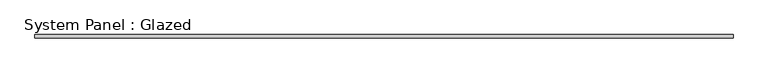
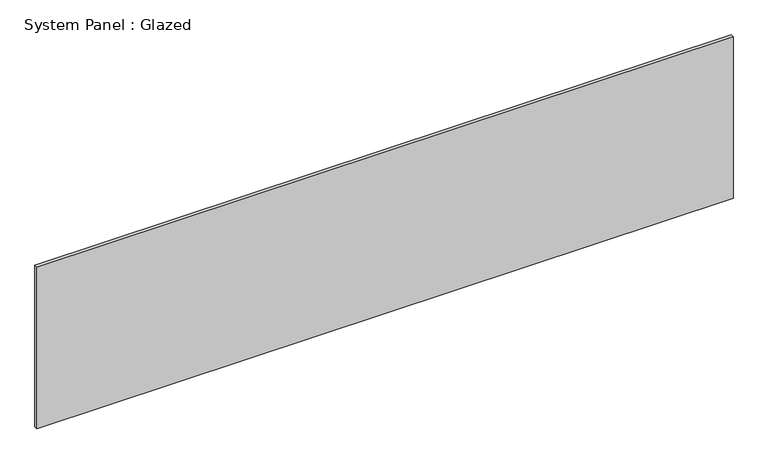
"""IFC4 building model written with IfcOpenShell, lengths in millimetres: plate geometry, System Panel : Glazed."""

from ifc_helpers import new_model, si_unit, origin, origin_with_axes, place, context, project, spatial, polyline, outline, extrude, source, transform, mapped, element, save


def system_panel_glazed_2422818d(model_context):
    return source(origin(), model_context, "Body", "SweptSolid", [
        extrude(outline(polyline([(2488.1784, 19.05), (-2488.1784, 19.05), (-2488.1784, 44.45), (2488.1784, 44.45), (2488.1784, 19.05)])), origin_with_axes(), (0.0, 0.0, 1.0), 1219.2),
    ])


if __name__ == "__main__":
    model = new_model("IFC4")
    model_context = context("Model", 3, world=origin())
    ifc_project = project(units=[si_unit("LENGTHUNIT", "METRE", prefix="MILLI")], contexts=[model_context])
    site = spatial("IfcSite", under=ifc_project)
    building = spatial("IfcBuilding", under=site)
    placement = place(None, origin())
    system_panel_glazed_shape = system_panel_glazed_2422818d(model_context)
    element("IfcPlate", 1, ObjectType="System Panel : Glazed", at=placement, inside=building, context=model_context, shape_type="MappedRepresentation", body=[
        mapped(system_panel_glazed_shape, transform((0.0, 0.0, 0.0), x_axis=(1.0, 0.0, 0.0), y_axis=(0.0, 1.0, 0.0), z_axis=(0.0, 0.0, 1.0))),
    ])
    save(model, "model.ifc")

# Revit data of these elements
# Type "System Panel : Glazed"
#   Construction Type Id = "GSP4R"
#   Analytic Construction = "1/8 in Pilkington single glazing"
#   Visual Light Transmittance = 0.9
#   Solar Heat Gain Coefficient = 0.86
#   Heat Transfer Coefficient (U) = 1.18115 BTU/(h·ft²·°F)
# Element 1 (IfcPlate, "System Panel : Glazed")
#   Materials on its faces: "Glass"
# Materials
#   "Glass": class "Glass", colour RGB 0 128 192, transparency 0.75, Description = "Soda Lime Glass", Cost = 0
